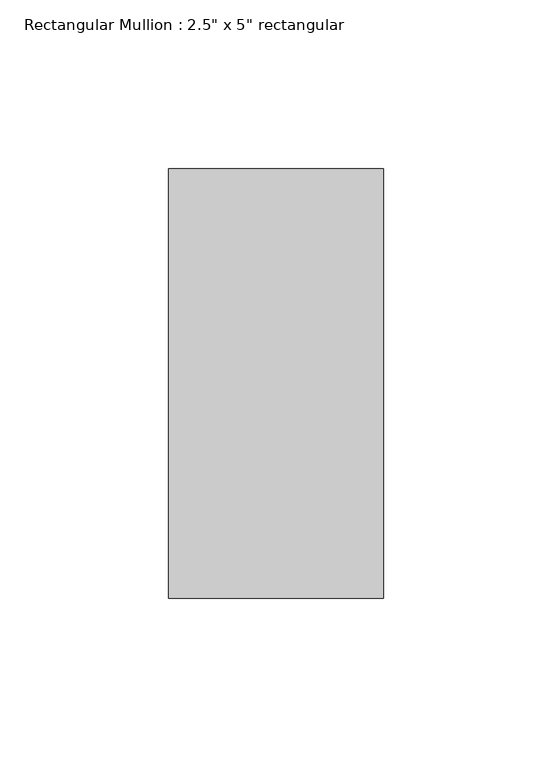
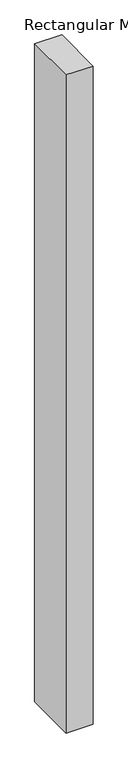
"""IFC4 building model written with IfcOpenShell, lengths in millimetres: member geometry."""

from ifc_helpers import new_model, si_unit, frame, origin, place, context, project, spatial, polyline, outline, extrude, source, transform, mapped, element, save


def member_80dcf73b(model_context):
    return source(origin(), model_context, "Body", "SweptSolid", [
        extrude(outline(polyline([(0.0, 63.5), (0.0, -63.5), (-63.5, -63.5), (-63.5, 63.5), (0.0, 63.5)])), frame((0.0, 0.0, -1629.9147167), z_axis=(0.0, 0.0, 1.0), x_axis=(1.0, 0.0, 0.0)), (0.0, 0.0, 1.0), 1629.9147167),
    ])


if __name__ == "__main__":
    model = new_model("IFC4")
    model_context = context("Model", 3, world=origin())
    ifc_project = project(units=[si_unit("LENGTHUNIT", "METRE", prefix="MILLI")], contexts=[model_context])
    site = spatial("IfcSite", under=ifc_project)
    building = spatial("IfcBuilding", under=site)
    placement = place(None, origin())
    member_shape = member_80dcf73b(model_context)
    element("IfcMember", 1, ObjectType="Rectangular Mullion : 2.5\" x 5\" rectangular", at=placement, inside=building, context=model_context, shape_type="MappedRepresentation", body=[
        mapped(member_shape, transform((0.0, 0.0, 0.0), x_axis=(1.0, 0.0, 0.0), y_axis=(0.0, 1.0, 0.0), z_axis=(0.0, 0.0, 1.0))),
    ])
    save(model, "model.ifc")

# Revit data of these elements
# Type "Rectangular Mullion : 2.5\" x 5\" rectangular"
#   built-in parameter 1007304 = 0.416667 (stored number, unit not read)
#   built-in parameter 1007301 = 0.104167 (stored number, unit not read)
#   built-in parameter 1007300 = 0.104167 (stored number, unit not read)
# Element 1 (IfcMember, "Rectangular Mullion : 2.5\" x 5\" rectangular")
#   Materials on its faces: "Aluminum"
# Materials
#   "Aluminum": class "Metal", colour RGB 247 247 247, transparency 0, Description = "Aluminum 6061", Cost = 0
